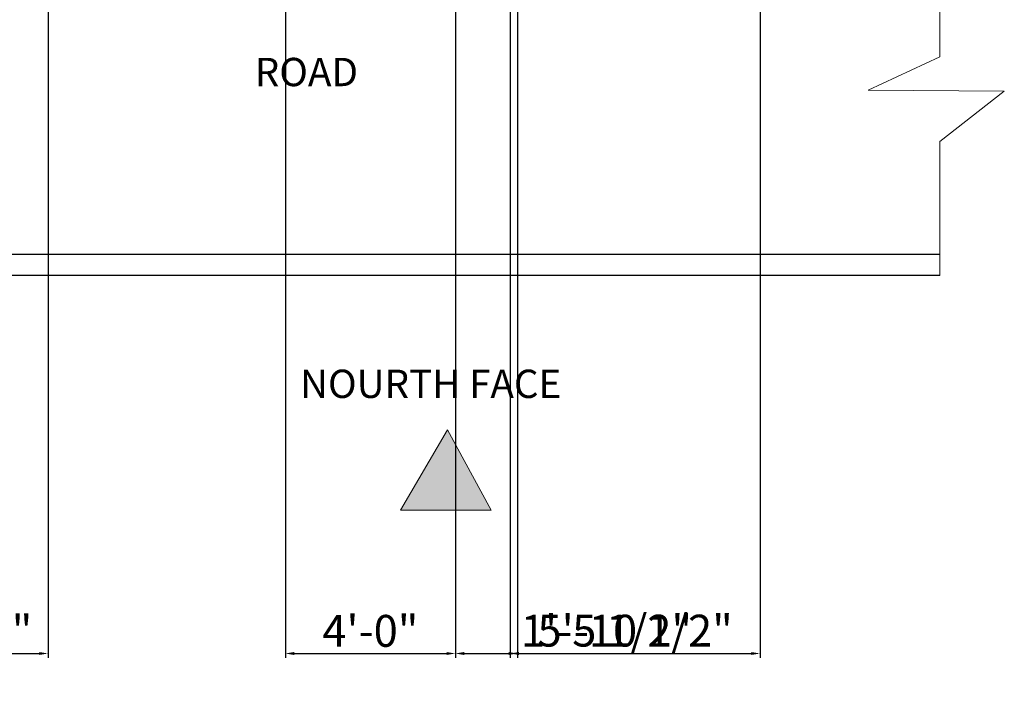
# Model space of a CAD drawing. Units: inches. Extents: x 635 to 1184, y 1837 to 2697.
# Tile 2 of 6: x 857 to 1135, y 1837 to 2024. Entities that reach past the tile are written whole.
import ezdxf

# ---------------------------------------------------------------- set-up
doc = ezdxf.new("R2010")
doc.units = ezdxf.units.IN
for name, color, linetype, lineweight in [('A-ANNO-DIMS', 2, 'Continuous', 18), ('A-ANNO-SYMB', 7, 'Continuous', 18), ('A-ANNO-TEXT', 7, 'Continuous', 25), ('C-ROAD', 8, 'Continuous', 25)]:
    doc.layers.add(name, color=color, linetype=linetype, lineweight=lineweight)
doc.styles.get("Standard").update_dxf_attribs({"font": 'arial.ttf'})
doc.dimstyles.new('ISO-25', dxfattribs={"dimtxt": 9, "dimasz": 2.5, "dimexe": 1.25, "dimexo": 0.625, "dimtad": 1, "dimlunit": 3, "dimtxsty": 'Standard', "dimcen": 2.5, "dimadec": 0, "dimazin": 0, "dimtfac": 1, "dimtmove": 0, "dimatfit": 3, "dimfxl": 1, "dimarcsym": 0})

# ---------------------------------------------------------------- blocks, each defined once
blk = doc.blocks.new('*D49')
at = {"layer": 'A-ANNO-DIMS', "color": 0, "lineweight": -2, "transparency": 16777216}
for p, q in [((932.28, 2155.52), (932.28, 1843.99)), ((980.28, 2155.52), (980.28, 1843.99)), ((934.78, 1845.24), (977.78, 1845.24))]:
    blk.add_line(p, q, dxfattribs=at)
at = {"layer": 'A-ANNO-DIMS', "color": 0, "transparency": 16777216}
for points in [[(934.78, 1845.65), (934.78, 1844.82), (932.28, 1845.24)], [(977.78, 1845.65), (977.78, 1844.82), (980.28, 1845.24)]]:
    blk.add_solid(points, dxfattribs=at)
at = {"layer": 'DEFPOINTS', "color": 0, "transparency": 16777216}
for p in [(932.28, 2156.14), (980.28, 2156.14), (980.28, 1845.24)]:
    blk.add_point(p, dxfattribs=at)
at = {"layer": 'A-ANNO-DIMS', "color": 0, "transparency": 16777216, "insert": (956.28, 1850.46), "char_height": 9, "attachment_point": 5}
blk.add_mtext('4\'-0"', dxfattribs=at)
blk = doc.blocks.new('*D50')
at = {"layer": 'A-ANNO-DIMS', "color": 0, "lineweight": -2, "transparency": 16777216}
for p, q in [((980.28, 2155.52), (980.28, 1843.99)), ((997.78, 2155.52), (997.78, 1843.99)), ((982.78, 1845.24), (995.28, 1845.24)), ((997.78, 1845.24), (1045.58, 1845.24))]:
    blk.add_line(p, q, dxfattribs=at)
at = {"layer": 'A-ANNO-DIMS', "color": 0, "transparency": 16777216}
for points in [[(982.78, 1845.65), (982.78, 1844.82), (980.28, 1845.24)], [(995.28, 1845.65), (995.28, 1844.82), (997.78, 1845.24)]]:
    blk.add_solid(points, dxfattribs=at)
at = {"layer": 'DEFPOINTS', "color": 0, "transparency": 16777216}
for p in [(980.28, 2156.14), (997.78, 2156.14), (997.78, 1845.24)]:
    blk.add_point(p, dxfattribs=at)
at = {"layer": 'A-ANNO-DIMS', "color": 0, "transparency": 16777216, "insert": (1022.93, 1850.52), "char_height": 9, "attachment_point": 5}
blk.add_mtext('1\'-5 1/2"', dxfattribs=at)
blk = doc.blocks.new('*D62')
at = {"layer": 'A-ANNO-DIMS', "color": 0, "lineweight": -2, "transparency": 16777216}
for p, q in [((829.28, 2442.52), (829.28, 1843.99)), ((865.28, 2442.52), (865.28, 1843.99)), ((831.78, 1845.24), (862.78, 1845.24))]:
    blk.add_line(p, q, dxfattribs=at)
at = {"layer": 'A-ANNO-DIMS', "color": 0, "transparency": 16777216}
for points in [[(831.78, 1845.65), (831.78, 1844.82), (829.28, 1845.24)], [(862.78, 1845.65), (862.78, 1844.82), (865.28, 1845.24)]]:
    blk.add_solid(points, dxfattribs=at)
at = {"layer": 'DEFPOINTS', "color": 0, "transparency": 16777216}
for p in [(829.28, 2443.14), (865.28, 2443.14), (865.28, 1845.24)]:
    blk.add_point(p, dxfattribs=at)
at = {"layer": 'A-ANNO-DIMS', "color": 0, "transparency": 16777216, "insert": (847.28, 1850.46), "char_height": 9, "attachment_point": 5}
blk.add_mtext('3\'-0"', dxfattribs=at)
blk = doc.blocks.new('*D63')
at = {"layer": 'A-ANNO-DIMS', "color": 0, "lineweight": -2, "transparency": 16777216}
for p, q in [((995.78, 2448.52), (995.78, 1843.99)), ((1066.28, 2448.52), (1066.28, 1843.99)), ((998.28, 1845.24), (1063.78, 1845.24))]:
    blk.add_line(p, q, dxfattribs=at)
at = {"layer": 'A-ANNO-DIMS', "color": 0, "transparency": 16777216}
for points in [[(998.28, 1845.65), (998.28, 1844.82), (995.78, 1845.24)], [(1063.78, 1845.65), (1063.78, 1844.82), (1066.28, 1845.24)]]:
    blk.add_solid(points, dxfattribs=at)
at = {"layer": 'DEFPOINTS', "color": 0, "transparency": 16777216}
for p in [(995.78, 2449.14), (1066.28, 2449.14), (1066.28, 1845.24)]:
    blk.add_point(p, dxfattribs=at)
at = {"layer": 'A-ANNO-DIMS', "color": 0, "transparency": 16777216, "insert": (1031.03, 1850.52), "char_height": 9, "attachment_point": 5}
blk.add_mtext('5\'-10 1/2"', dxfattribs=at)

msp = doc.modelspace()

# ---------------------------------------------------------------- hatches: boundary and pattern name
at = {"layer": 'A-ANNO-SYMB'}
h = msp.add_hatch(color=256, dxfattribs=at)
h.dxf.hatch_style = 1
h.paths.add_polyline_path([(978.007, 1908.412), (964.784, 1885.737), (990.387, 1885.737)])
h.paths.add_polyline_path([(747.282, 2339.586), (738.604, 2324.556), (746.882, 2324.556), (746.882, 2322.142), (747.682, 2322.142), (747.682, 2324.556), (755.96, 2324.556)])

# ---------------------------------------------------------------- linework, layer by layer
msp.add_lwpolyline([(1117.034, 2059.142), (1117.034, 2013.802), (1096.782, 2004.337), (1135.238, 2004.087), (1117.034, 1989.817), (1117.034, 1951.962)], dxfattribs=at)
msp.add_lwpolyline([(978.007, 1908.412), (964.784, 1885.737), (990.387, 1885.737)], close=True, dxfattribs=at)
at = {"layer": 'C-ROAD'}
for p, q in [((1117.034, 1957.962), (714.282, 1957.962)), ((1117.034, 1951.962), (714.282, 1951.962))]:
    msp.add_line(p, q, dxfattribs=at)

# ---------------------------------------------------------------- texts
at = {"layer": 'A-ANNO-TEXT', "char_height": 8, "attachment_point": 1}
for s, width, insert in [('ROAD', 32.94677, (923.627, 2013.475)), ('NOURTH FACE ', 85.76437, (936.421, 1925.406))]:
    msp.add_mtext_dynamic_manual_height_columns(s, width=width, gutter_width=12.5, heights=[0], dxfattribs=dict(at, insert=insert))

# ---------------------------------------------------------------- dimensions: what is measured, and where the dimension line sits
at = {"layer": 'A-ANNO-DIMS'}
for base, p1, p2, picture, middle in [((1066.282, 1845.237), (995.782, 2449.142), (1066.282, 2449.142), '*D63', (1031.032, 1850.516)), ((865.282, 1845.237), (829.282, 2443.142), (865.282, 2443.142), '*D62', (847.282, 1850.461)), ((980.282, 1845.237), (932.282, 2156.142), (980.282, 2156.142), '*D49', (956.282, 1850.458)), ((997.782, 1845.237), (980.282, 2156.142), (997.782, 2156.142), '*D50', (1022.931, 1850.516))]:
    dim = msp.add_linear_dim(base=base, p1=p1, p2=p2, dimstyle='ISO-25', override={"dimdec": 1, "dimlfac": 1, "dimrnd": 0, "dimzin": 1, "dimdsep": 46, "dimlunit": 4, "dimfrac": 2}, dxfattribs=at)
    dim.commit()
    dim.dimension.update_dxf_attribs({"geometry": picture, "text_midpoint": middle})

doc.saveas('drawing.dxf')
